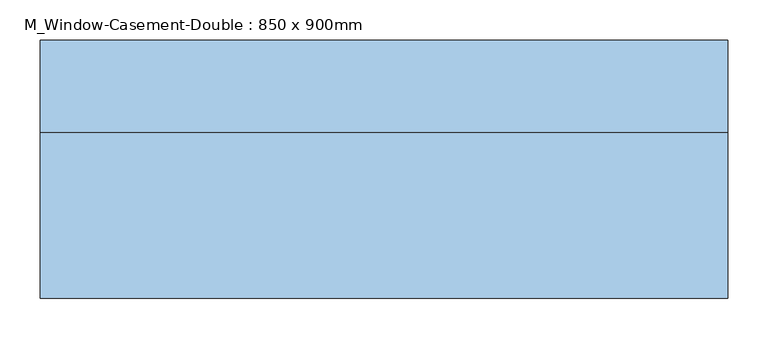
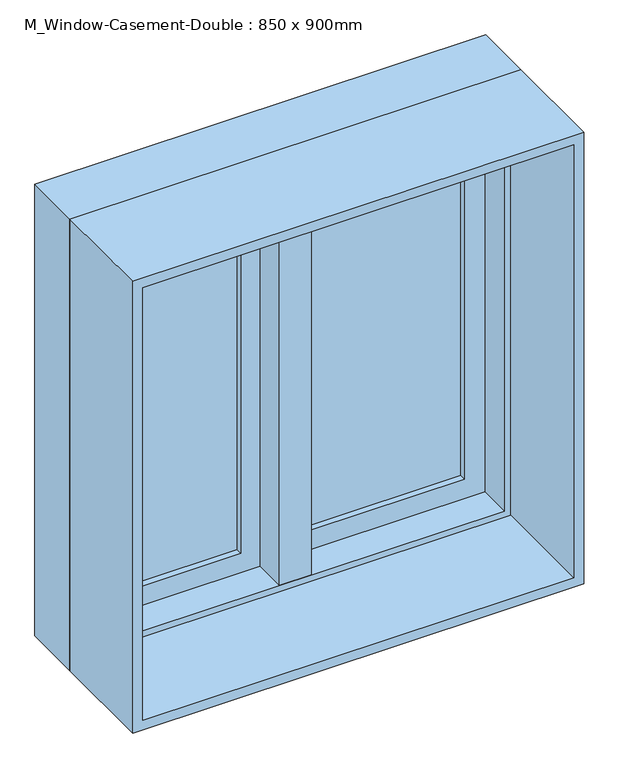
"""IFC4 building model written with IfcOpenShell, lengths in millimetres: window geometry, M_Window-Casement-Double : 850 x 900mm."""

from ifc_helpers import new_model, si_unit, frame, origin, place, context, project, spatial, polyline, outline, extrude, faceted_brep, source, transform, mapped, element, save


def m_window_casement_double_850_x_900mm_d87c3818(model_context):
    return source(origin(), model_context, "Body", "SolidModel", [
        faceted_brep([(9.525, 169.05, 1787.3), (-9.525, 169.05, 1787.3), (-9.525, 118.25, 1787.3), (9.525, 118.25, 1787.3), (9.525, 169.05, 912.7), (9.525, 118.25, 912.7), (-9.525, 118.25, 912.7), (-9.525, 169.05, 912.7), (-9.525, 118.25, 931.75), (-9.525, 118.25, 1768.25), (-30.1625, 118.25, 931.75), (-30.1625, 118.25, 1768.25), (-30.1625, 54.75, 931.75), (-30.1625, 54.75, 1768.25), (30.1625, 54.75, 931.75), (30.1625, 54.75, 1768.25), (30.1625, 118.25, 931.75), (30.1625, 118.25, 1768.25), (9.525, 118.25, 931.75), (9.525, 118.25, 1768.25)], [[[0, 1, 2, 3]], [[4, 5, 6, 7]], [[1, 0, 4, 7]], [[2, 1, 7, 6, 8, 9]], [[9, 8, 10, 11]], [[11, 10, 12, 13]], [[13, 12, 14, 15]], [[15, 14, 16, 17]], [[17, 16, 18, 19]], [[0, 3, 19, 18, 5, 4]], [[18, 8, 6, 5]], [[9, 19, 3, 2]], [[8, 18, 16, 14, 12, 10]], [[19, 9, 11, 13, 15, 17]]]),
        extrude(outline(polyline([(-66.675, 150.0), (-66.675, 143.65), (-355.15, 143.65), (-355.15, 150.0), (-66.675, 150.0)])), frame((0.0, 0.0, 969.85), z_axis=(0.0, 0.0, 1.0), x_axis=(1.0, 0.0, 0.0)), (0.0, 0.0, 1.0), 760.3),
        extrude(outline(polyline([(-355.15, 130.95), (-355.15, 137.3), (-66.675, 137.3), (-66.675, 130.95), (-355.15, 130.95)])), frame((0.0, 0.0, 969.85), z_axis=(0.0, 0.0, 1.0), x_axis=(1.0, 0.0, 0.0)), (0.0, 0.0, 1.0), 760.3),
        extrude(outline(polyline([(355.15, 150.0), (355.15, 143.65), (66.675, 143.65), (66.675, 150.0), (355.15, 150.0)])), frame((0.0, 0.0, 969.85), z_axis=(0.0, 0.0, 1.0), x_axis=(1.0, 0.0, 0.0)), (0.0, 0.0, 1.0), 760.3),
        extrude(outline(polyline([(66.675, 130.95), (66.675, 137.3), (355.15, 137.3), (355.15, 130.95), (66.675, 130.95)])), frame((0.0, 0.0, 969.85), z_axis=(0.0, 0.0, 1.0), x_axis=(1.0, 0.0, 0.0)), (0.0, 0.0, 1.0), 760.3),
        extrude(outline(polyline([(1787.3, -412.3), (912.7, -412.3), (912.7, -9.525), (1787.3, -9.525), (1787.3, -412.3)]), holes=[polyline([(1730.15, -66.675), (969.85, -66.675), (969.85, -355.15), (1730.15, -355.15), (1730.15, -66.675)])]), frame((0.0, 118.25, 0.0), z_axis=(0.0, 1.0, 0.0), x_axis=(0.0, 0.0, 1.0)), (0.0, 0.0, 1.0), 44.45),
        extrude(outline(polyline([(912.7, 412.3), (1787.3, 412.3), (1787.3, 9.525), (912.7, 9.525), (912.7, 412.3)]), holes=[polyline([(969.85, 66.675), (1730.15, 66.675), (1730.15, 355.15), (969.85, 355.15), (969.85, 66.675)])]), frame((0.0, 118.25, 0.0), z_axis=(0.0, 1.0, 0.0), x_axis=(0.0, 0.0, 1.0)), (0.0, 0.0, 1.0), 44.45),
        extrude(outline(polyline([(1800.0, -425.0), (900.0, -425.0), (900.0, 425.0), (1800.0, 425.0), (1800.0, -425.0)]), holes=[polyline([(1780.95, 405.95), (919.05, 405.95), (919.05, -405.95), (1780.95, -405.95), (1780.95, 405.95)])]), frame((0.0, -150.0, 0.0), z_axis=(0.0, 1.0, 0.0), x_axis=(0.0, 0.0, 1.0)), (0.0, 0.0, 1.0), 204.75),
        faceted_brep([(393.25, 118.25, 1768.25), (393.25, 54.75, 1768.25), (-393.25, 54.75, 1768.25), (-393.25, 118.25, 1768.25), (412.3, 169.05, 1787.3), (412.3, 118.25, 1787.3), (-412.3, 118.25, 1787.3), (-412.3, 169.05, 1787.3), (425.0, 54.75, 1800.0), (425.0, 169.05, 1800.0), (-425.0, 169.05, 1800.0), (-425.0, 54.75, 1800.0), (-393.25, 54.75, 931.75), (-393.25, 118.25, 931.75), (-412.3, 118.25, 912.7), (-412.3, 169.05, 912.7), (-425.0, 169.05, 900.0), (-425.0, 54.75, 900.0), (393.25, 54.75, 931.75), (393.25, 118.25, 931.75), (412.3, 118.25, 912.7), (412.3, 169.05, 912.7), (425.0, 169.05, 900.0), (425.0, 54.75, 900.0)], [[[0, 1, 2, 3]], [[4, 5, 6, 7]], [[8, 9, 10, 11]], [[3, 2, 12, 13]], [[7, 6, 14, 15]], [[11, 10, 16, 17]], [[13, 12, 18, 19]], [[15, 14, 20, 21]], [[17, 16, 22, 23]], [[11, 17, 23, 8], [1, 18, 12, 2]], [[19, 18, 1, 0]], [[5, 20, 14, 6], [3, 13, 19, 0]], [[21, 20, 5, 4]], [[23, 22, 9, 8]], [[9, 22, 16, 10], [7, 15, 21, 4]]]),
    ])


if __name__ == "__main__":
    model = new_model("IFC4")
    model_context = context("Model", 3, world=origin())
    ifc_project = project(units=[si_unit("LENGTHUNIT", "METRE", prefix="MILLI")], contexts=[model_context])
    site = spatial("IfcSite", under=ifc_project)
    building = spatial("IfcBuilding", under=site)
    placement = place(None, origin())
    m_window_casement_double_850_x_900mm_shape = m_window_casement_double_850_x_900mm_d87c3818(model_context)
    element("IfcWindow", 1, ObjectType="M_Window-Casement-Double : 850 x 900mm", at=placement, inside=building, context=model_context, shape_type="MappedRepresentation", body=[
        mapped(m_window_casement_double_850_x_900mm_shape, transform((0.0, 0.0, 0.0), x_axis=(1.0, 0.0, 0.0), y_axis=(0.0, 1.0, 0.0), z_axis=(0.0, 0.0, 1.0))),
    ])
    save(model, "model.ifc")

# Revit data of these elements
# Type "M_Window-Casement-Double : 850 x 900mm"
#   Type Mark = "23"
#   Fire Rating = "0.5h"
#   Assembly Code = "B2020100"
#   Analytic Construction = "Double glazing - domestic"
#   Frame Extension [instance default] = 6.35 mm
#   Window Inset [instance default] = 0 mm
#   Wall Thickness [instance default] = 150 mm
#   Interior Wall Closure [instance default] = 54.75 mm
#   Half Width = 425 mm
#   Visual Light Transmittance = 0.81
#   Thermal Resistance (R) = 0.319569 (m²·K)/W
#   Solar Heat Gain Coefficient = 0.76
#   Rough Width = 865 mm
#   Rough Height = 915 mm
#   Height = 900 mm
#   Heat Transfer Coefficient (U) = 3.12929 W/(m²·K)
#   Exterior Wall Closure [instance default] = 31.8 mm
#   Extension Jamb [instance default] = 54.75 mm
#   Default Sill Height = 900 mm
#   Width = 850 mm
#   Define Thermal Properties by = 0
#   Muntin Visibility = yes
#   Interior Trim Visibility [instance default] = yes
#   Exterior Trim Visibility [instance default] = yes
#   Extension Jamb Visibility [instance default] = yes
#   Interior Trim Material = Wood - Stained
#   Muntin Pattern = M_Muntin Pattern_2x2 : M_Muntin Pattern_2x2
#   Interior Trim = M_Trim-Window-Interior-Flat : Picture Frame
#   Interior Frame Material = Wood - Stained
#   Glass Panel Material = Glass
#   Exterior Trim Material = Clad - White
#   Exterior Trim = M_Trim-Window-Exterior-Flat : with Sill
#   Exterior Frame Material = Clad - White
#   Wall Closure = (empty or 0)
# Element 1 (IfcWindow, "M_Window-Casement-Double : 850 x 900mm")
#   Wall Thickness = 300 mm
#   Extension Jamb = 204.75 mm
#   Materials on its faces: "Wood - Stained", "Glass", "Clad - White"
# Materials
#   "Wood - Stained": class "Wood", colour RGB 224 178 126, transparency 0, Cost = 0
#   "Glass": class "Glass", colour RGB 0 128 192, transparency 0.9, Description = "Soda Lime Glass", Cost = 0
#   "Clad - White": class "Wood", colour RGB 242 242 238, transparency 0, Cost = 0
